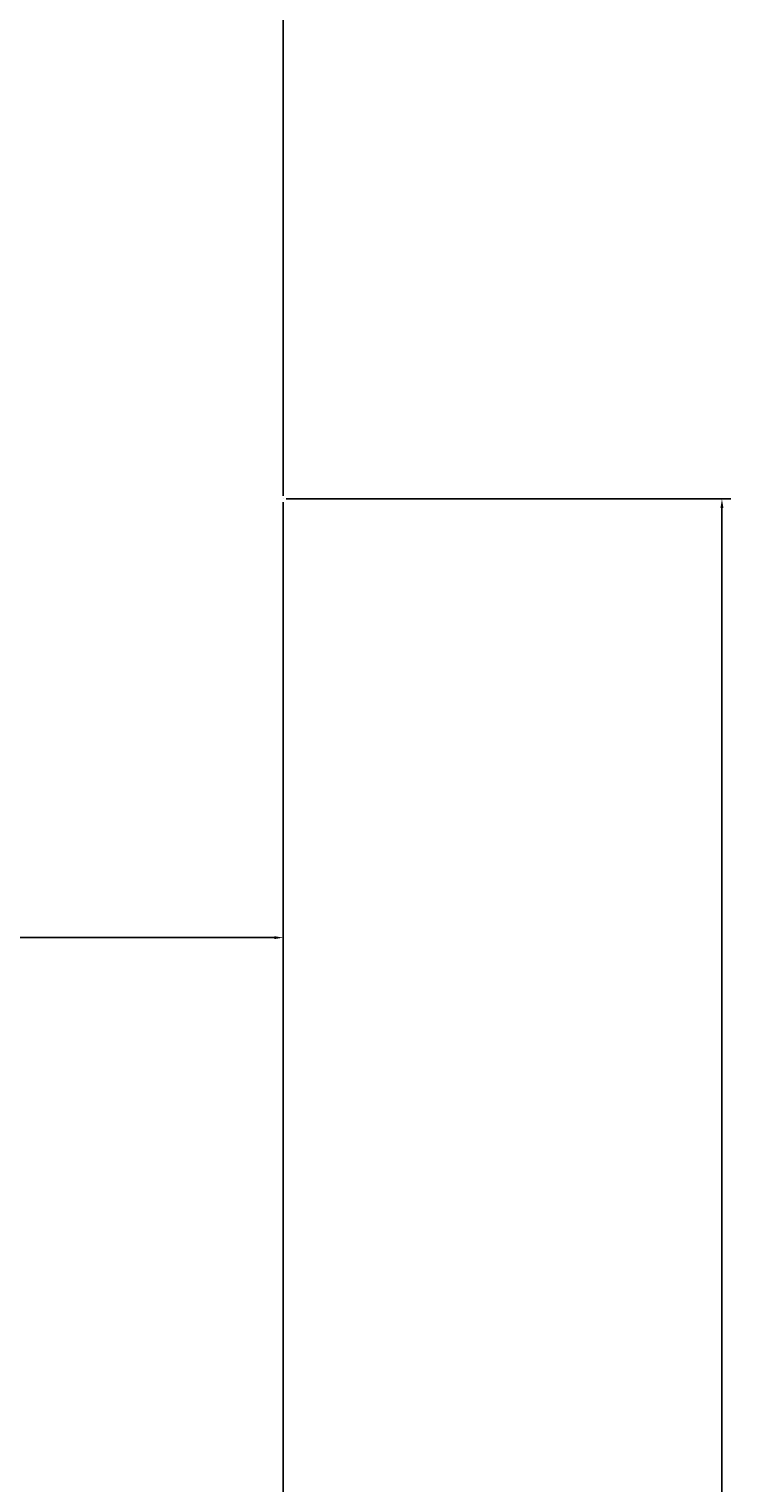
# Model space of a CAD drawing. Units: millimetres. Extents: x -9 to 135, y -119 to 27.
# Tile 11 of 12: x 121 to 135, y -18 to 11. Entities that reach past the tile are written whole.
import ezdxf

# ---------------------------------------------------------------- set-up
doc = ezdxf.new("R2010")
doc.units = ezdxf.units.MM
doc.layers.add('M-CONS', color=8, linetype='Continuous', lineweight=18)
doc.layers.add('M-DIMS', color=2, linetype='Continuous', lineweight=18)
doc.styles.get("Standard").update_dxf_attribs({"font": 'arial.ttf'})
doc.dimstyles.get("Standard").update_dxf_attribs({"dimtxt": 0.18, "dimasz": 0.18, "dimexe": 0.18, "dimexo": 0.0625, "dimgap": 0.09, "dimtad": 0, "dimtih": 1, "dimtoh": 1, "dimdec": 4, "dimzin": 0, "dimdsep": 46, "dimtxsty": 'Standard', "dimcen": 0.09, "dimadec": 0, "dimazin": 0, "dimtfac": 1, "dimtdec": 4, "dimtofl": 0, "dimtmove": 0, "dimatfit": 3, "dimfxl": 1, "dimtolj": 1, "dimtzin": 0, "dimarcsym": 0})

# ---------------------------------------------------------------- blocks, each defined once
blk = doc.blocks.new('*D2')
at = {"layer": 'Defpoints', "color": 0, "transparency": 16777216}
for p in [(126, 26.533), (0, 17.733), (126, 1.733)]:
    blk.add_point(p, dxfattribs=at)
at = {"layer": 'M-DIMS', "color": 0, "lineweight": -2, "transparency": 16777216}
for p, q in [((0, 17.796), (0, 26.713)), ((126, 1.796), (126, 26.713)), ((0.18, 26.533), (62.72, 26.533)), ((125.82, 26.533), (63.28, 26.533))]:
    blk.add_line(p, q, dxfattribs=at)
at = {"layer": 'M-DIMS', "color": 0, "transparency": 16777216}
for points in [[(0.18, 26.563), (0.18, 26.503), (0, 26.533)], [(125.82, 26.563), (125.82, 26.503), (126, 26.533)]]:
    blk.add_solid(points, dxfattribs=at)
at = {"layer": 'M-DIMS', "color": 0, "transparency": 16777216, "insert": (63, 26.533), "char_height": 0.18, "attachment_point": 5}
blk.add_mtext('\\A1;126', dxfattribs=at)
blk = doc.blocks.new('*D11')
at = {"layer": 'Defpoints', "color": 0, "transparency": 16777216}
for p in [(108, 1.733), (126, 1.733), (108, -7.067)]:
    blk.add_point(p, dxfattribs=at)
at = {"layer": 'M-DIMS', "color": 0, "lineweight": -2, "transparency": 16777216}
for p, q in [((108, 1.671), (108, -7.247)), ((126, 1.671), (126, -7.247)), ((108.18, -7.067), (116.789, -7.067)), ((125.82, -7.067), (117.211, -7.067))]:
    blk.add_line(p, q, dxfattribs=at)
at = {"layer": 'M-DIMS', "color": 0, "transparency": 16777216}
for points in [[(108.18, -7.037), (108.18, -7.097), (108, -7.067)], [(125.82, -7.037), (125.82, -7.097), (126, -7.067)]]:
    blk.add_solid(points, dxfattribs=at)
at = {"layer": 'M-DIMS', "color": 0, "transparency": 16777216, "insert": (117, -7.067), "char_height": 0.18, "attachment_point": 5}
blk.add_mtext('\\A1;18', dxfattribs=at)
blk = doc.blocks.new('*D13')
at = {"layer": 'Defpoints', "color": 0, "transparency": 16777216}
for p in [(126, 1.733), (63, -92.267), (134.8, -92.267)]:
    blk.add_point(p, dxfattribs=at)
at = {"layer": 'M-DIMS', "color": 0, "lineweight": -2, "transparency": 16777216}
for p, q in [((126.062, 1.733), (134.98, 1.733)), ((134.8, 1.553), (134.8, -45.085)), ((134.8, -92.087), (134.8, -45.449)), ((63.063, -92.267), (134.98, -92.267))]:
    blk.add_line(p, q, dxfattribs=at)
at = {"layer": 'M-DIMS', "color": 0, "transparency": 16777216}
for points in [[(134.77, 1.553), (134.83, 1.553), (134.8, 1.733)], [(134.77, -92.087), (134.83, -92.087), (134.8, -92.267)]]:
    blk.add_solid(points, dxfattribs=at)
at = {"layer": 'M-DIMS', "color": 0, "transparency": 16777216, "insert": (134.8, -45.267), "char_height": 0.18, "attachment_point": 5}
blk.add_mtext('\\A1;94', dxfattribs=at)
blk = doc.blocks.new('*D16')
at = {"layer": 'Defpoints', "color": 0, "transparency": 16777216}
for p in [(126, 1.733), (63, -92.267), (126, -119.067)]:
    blk.add_point(p, dxfattribs=at)
at = {"layer": 'M-DIMS', "color": 0, "lineweight": -2, "transparency": 16777216}
for p, q in [((126, 1.671), (126, -119.247)), ((63, -92.329), (63, -119.247)), ((63.18, -119.067), (94.281, -119.067)), ((125.82, -119.067), (94.719, -119.067))]:
    blk.add_line(p, q, dxfattribs=at)
at = {"layer": 'M-DIMS', "color": 0, "transparency": 16777216}
for points in [[(63.18, -119.037), (63.18, -119.097), (63, -119.067)], [(125.82, -119.037), (125.82, -119.097), (126, -119.067)]]:
    blk.add_solid(points, dxfattribs=at)
at = {"layer": 'M-DIMS', "color": 0, "transparency": 16777216, "insert": (94.5, -119.067), "char_height": 0.18, "attachment_point": 5}
blk.add_mtext('\\A1;63', dxfattribs=at)

msp = doc.modelspace()

# ---------------------------------------------------------------- linework, layer by layer
at = {"layer": 'M-CONS', "extrusion": (0, -1, 0)}
msp.add_line((126, 1.733, 71.129), (126, 1.733, 101.129), dxfattribs=at)

# ---------------------------------------------------------------- dimensions: what is measured, and where the dimension line sits
at = {"layer": 'M-DIMS'}
for base, p1, picture, middle in [((126, 26.533), (0, 17.733), '*D2', (63, 26.533)), ((126, -119.067), (63, -92.267), '*D16', (94.5, -119.067))]:
    dim = msp.add_linear_dim(base=base, p1=p1, p2=(126, 1.733), dimstyle='Standard', override={"dimdec": 0, "dimlfac": 1, "dimrnd": 0, "dimzin": 0, "dimdsep": 46, "dimlunit": 2}, dxfattribs=at)
    dim.commit()
    dim.dimension.update_dxf_attribs({"geometry": picture, "text_midpoint": middle})
for base, p2, angle, picture, middle in [((134.8, -92.267), (63, -92.267), 90, '*D13', (134.8, -45.267)), ((108, -7.067), (108, 1.733), 180, '*D11', (117, -7.067))]:
    dim = msp.add_linear_dim(base=base, p1=(126, 1.733), p2=p2, angle=angle, dimstyle='Standard', override={"dimdec": 0, "dimlfac": 1, "dimrnd": 0, "dimzin": 0, "dimdsep": 46, "dimlunit": 2}, dxfattribs=at)
    dim.commit()
    dim.dimension.update_dxf_attribs({"geometry": picture, "text_midpoint": middle})

doc.saveas('drawing.dxf')
